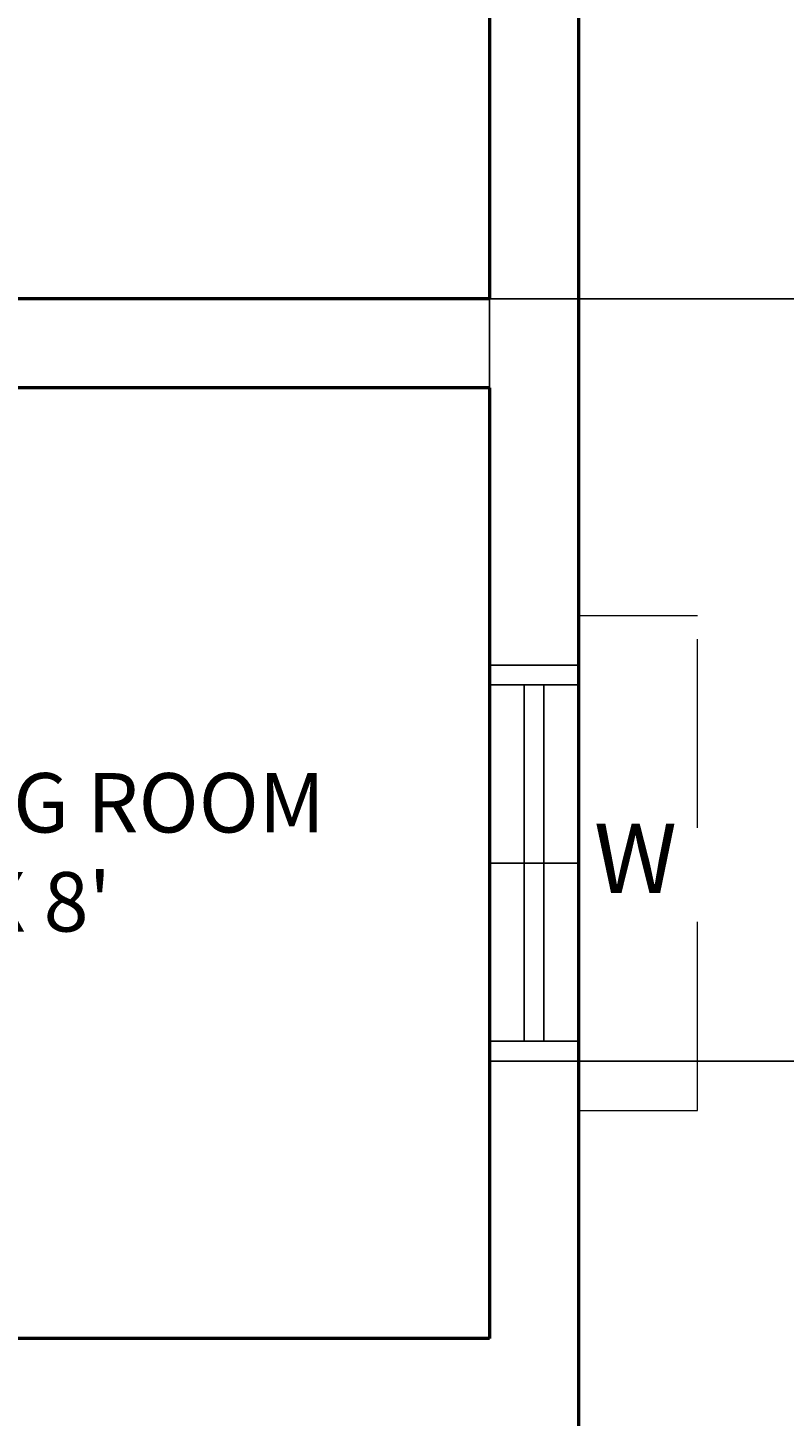
# Model space of a CAD drawing. Units: inches. Extents: x 37 to 824, y -700 to 234.
# Tile 40 of 77: x 372 to 449, y -215 to -75. Entities that reach past the tile are written whole.
import ezdxf

# ---------------------------------------------------------------- set-up
doc = ezdxf.new("R2010")
doc.units = ezdxf.units.IN
doc.header["$MEASUREMENT"] = 0
doc.linetypes.add('DASHED', pattern=[19.05, 12.7, -6.35])
for name, color, linetype, lineweight in [('A-ANNO-DIMS', 2, 'Continuous', 18), ('A-ANNO-TEXT', 7, 'Continuous', 18), ('A-AREA-IDEN', 3, 'Continuous', 18), ('A-GLAZ', 4, 'Continuous', 25), ('A-ROOF-OVHD', 1, 'DASHED', 18), ('A-WALL', 2, 'Continuous', 50)]:
    doc.layers.add(name, color=color, linetype=linetype, lineweight=lineweight)
doc.styles.get("Standard").update_dxf_attribs({"font": 'arial.ttf'})
doc.dimstyles.get("Standard").update_dxf_attribs({"dimtxt": 0.18, "dimasz": 0.18, "dimexe": 0.18, "dimexo": 0.0625, "dimgap": 0.09, "dimtad": 0, "dimtih": 1, "dimtoh": 1, "dimdec": 1, "dimzin": 0, "dimdsep": 46, "dimlunit": 4, "dimtxsty": 'Standard', "dimcen": 0.09, "dimadec": 0, "dimazin": 0, "dimtfac": 1, "dimtdec": 1, "dimtofl": 0, "dimtmove": 0, "dimatfit": 3, "dimfxl": 1, "dimtolj": 1, "dimtzin": 0, "dimarcsym": 0})

# ---------------------------------------------------------------- blocks, each defined once
blk = doc.blocks.new('WIN-900')
for p, q in [((0, 9), (0, 0)), ((2, 9), (2, 0)), ((20, 9), (20, 0)), ((38, 9), (38, 0)), ((40, 9), (40, 0)), ((38, 5.5), (2, 5.5)), ((38, 3.5), (2, 3.5))]:
    blk.add_line(p, q)
blk = doc.blocks.new('*D64')
at = {"layer": 'A-ANNO-DIMS', "color": 0, "lineweight": -2, "ltscale": 0.5, "transparency": 16777216}
for p, q in [((428.14, 191.09), (513.77, 191.09)), ((513.59, 190.91), (513.59, -87.23)), ((513.59, -365.73), (513.59, -87.59)), ((428.14, -365.91), (513.77, -365.91))]:
    blk.add_line(p, q, dxfattribs=at)
at = {"layer": 'A-ANNO-DIMS', "color": 0, "ltscale": 0.5, "transparency": 16777216}
for points in [[(513.56, 190.91), (513.62, 190.91), (513.59, 191.09)], [(513.56, -365.73), (513.62, -365.73), (513.59, -365.91)]]:
    blk.add_solid(points, dxfattribs=at)
at = {"layer": 'Defpoints', "color": 0, "ltscale": 0.5, "transparency": 16777216}
for p in [(428.08, 191.09), (428.08, -365.91), (513.59, -365.91)]:
    blk.add_point(p, dxfattribs=at)
at = {"layer": 'A-ANNO-DIMS', "color": 0, "ltscale": 0.5, "transparency": 16777216, "insert": (513.59, -87.41), "char_height": 0.18, "attachment_point": 5}
blk.add_mtext('\\A1;46\'-5"', dxfattribs=at)
blk = doc.blocks.new('*D65')
at = {"layer": 'A-ANNO-DIMS', "color": 0, "lineweight": -2, "ltscale": 0.5, "transparency": 16777216}
for p, q in [((428.14, -178.91), (513.77, -178.91)), ((513.59, -179.09), (513.59, -272.23)), ((513.59, -365.73), (513.59, -272.59)), ((428.14, -365.91), (513.77, -365.91))]:
    blk.add_line(p, q, dxfattribs=at)
at = {"layer": 'A-ANNO-DIMS', "color": 0, "ltscale": 0.5, "transparency": 16777216}
for points in [[(513.56, -179.09), (513.62, -179.09), (513.59, -178.91)], [(513.56, -365.73), (513.62, -365.73), (513.59, -365.91)]]:
    blk.add_solid(points, dxfattribs=at)
at = {"layer": 'Defpoints', "color": 0, "ltscale": 0.5, "transparency": 16777216}
for p in [(428.08, -178.91), (428.08, -365.91), (513.59, -365.91)]:
    blk.add_point(p, dxfattribs=at)
at = {"layer": 'A-ANNO-DIMS', "color": 0, "ltscale": 0.5, "transparency": 16777216, "insert": (513.59, -272.41), "char_height": 0.18, "attachment_point": 5}
blk.add_mtext('\\A1;15\'-7"', dxfattribs=at)
blk = doc.blocks.new('*D79')
at = {"layer": 'A-ANNO-DIMS', "color": 0, "lineweight": -2, "ltscale": 0.5, "transparency": 16777216}
for p, q in [((299.14, -62.02), (513.77, -62.02)), ((513.59, -62.2), (513.59, -81.78)), ((513.59, -101.73), (513.59, -82.15)), ((296.14, -101.91), (513.77, -101.91))]:
    blk.add_line(p, q, dxfattribs=at)
at = {"layer": 'A-ANNO-DIMS', "color": 0, "ltscale": 0.5, "transparency": 16777216}
for points in [[(513.56, -62.2), (513.62, -62.2), (513.59, -62.02)], [(513.56, -101.73), (513.62, -101.73), (513.59, -101.91)]]:
    blk.add_solid(points, dxfattribs=at)
at = {"layer": 'Defpoints', "color": 0, "ltscale": 0.5, "transparency": 16777216}
for p in [(299.08, -62.02), (296.08, -101.91), (513.59, -101.91)]:
    blk.add_point(p, dxfattribs=at)
at = {"layer": 'A-ANNO-DIMS', "color": 0, "ltscale": 0.5, "transparency": 16777216, "insert": (513.59, -81.97), "char_height": 0.18, "attachment_point": 5}
blk.add_mtext('\\A1;3\'-4"', dxfattribs=at)
blk = doc.blocks.new('*D83')
at = {"layer": 'A-ANNO-DIMS', "color": 0, "lineweight": -2, "ltscale": 0.5, "transparency": 16777216}
for p, q in [((358.13, -206.85), (358.13, 234.17)), ((358.31, 233.99), (388.28, 233.99)), ((418.9, 233.99), (388.93, 233.99)), ((419.08, -206.85), (419.08, 234.17))]:
    blk.add_line(p, q, dxfattribs=at)
at = {"layer": 'A-ANNO-DIMS', "color": 0, "ltscale": 0.5, "transparency": 16777216}
for points in [[(358.31, 234.02), (358.31, 233.96), (358.13, 233.99)], [(418.9, 234.02), (418.9, 233.96), (419.08, 233.99)]]:
    blk.add_solid(points, dxfattribs=at)
at = {"layer": 'Defpoints', "color": 0, "ltscale": 0.5, "transparency": 16777216}
for p in [(419.08, 233.99), (358.13, -206.91), (419.08, -206.91)]:
    blk.add_point(p, dxfattribs=at)
at = {"layer": 'A-ANNO-DIMS', "color": 0, "ltscale": 0.5, "transparency": 16777216, "insert": (388.6, 233.99), "char_height": 0.18, "attachment_point": 5}
blk.add_mtext('\\A1;5\'-1"', dxfattribs=at)

msp = doc.modelspace()

# ---------------------------------------------------------------- linework, layer by layer
at = {"layer": 'A-ROOF-OVHD', "ltscale": 1.5}
for p, q in [((428.08, -138.91), (428.08, -133.91)), ((428.08, -133.91), (440.08, -133.91)), ((440.08, -183.91), (440.08, -133.91)), ((428.08, -178.91), (428.08, -183.91)), ((428.08, -183.91), (440.08, -183.91))]:
    msp.add_line(p, q, dxfattribs=at)
at = {"layer": 'A-WALL'}
for p, q in [((419.08, 6.09), (419.08, -101.91)), ((428.08, 6.09), (428.08, -110.91)), ((419.08, -101.91), (290.08, -101.91)), ((419.08, -110.91), (290.08, -110.91)), ((419.08, -110.91), (419.08, -206.91)), ((428.08, -110.91), (428.08, -215.91)), ((419.08, -206.91), (358.13, -206.91))]:
    msp.add_line(p, q, dxfattribs=at)

# ---------------------------------------------------------------- block references
at = {"layer": 'A-GLAZ', "rotation": 270.0000000000001}
msp.add_blockref('WIN-900', (419.08, -138.91), dxfattribs=at)

# ---------------------------------------------------------------- texts
at = {"layer": 'A-ANNO-TEXT'}
msp.add_text('W', height=7, dxfattribs=at).set_placement((429.63, -161.94))
at = {"layer": 'A-AREA-IDEN', "insert": (339.67, -149.82), "char_height": 6, "attachment_point": 1}
msp.add_mtext_dynamic_manual_height_columns("DRAWING ROOM\\P        10' X 8'", width=88.3217, gutter_width=1, heights=[0], dxfattribs=at)

# ---------------------------------------------------------------- dimensions: what is measured, and where the dimension line sits
at = {"layer": 'A-ANNO-DIMS', "ltscale": 0.5}
dim = msp.add_linear_dim(base=(419.0772, 233.9904), p1=(358.1323, -206.9096), p2=(419.0772, -206.9096), dimstyle='Standard', override={"dimdec": 1, "dimlfac": 1, "dimrnd": 0, "dimzin": 1, "dimdsep": 46, "dimlunit": 4, "dimfrac": 2}, dxfattribs=at)
dim.commit()
dim.dimension.update_dxf_attribs({"geometry": '*D83', "text_midpoint": (388.6047, 233.9904)})
for base, p1, p2, picture, middle in [((513.59, -365.91), (428.08, 191.09), (428.08, -365.91), '*D64', (513.59, -87.41)), ((513.59, -101.91), (299.08, -62.02), (296.08, -101.91), '*D79', (513.59, -81.97)), ((513.59, -365.91), (428.08, -178.91), (428.08, -365.91), '*D65', (513.59, -272.41))]:
    dim = msp.add_linear_dim(base=base, p1=p1, p2=p2, angle=90, dimstyle='Standard', override={"dimdec": 1, "dimlfac": 1, "dimrnd": 0, "dimzin": 1, "dimdsep": 46, "dimlunit": 4, "dimfrac": 2}, dxfattribs=at)
    dim.commit()
    dim.dimension.update_dxf_attribs({"geometry": picture, "text_midpoint": middle})

doc.saveas('drawing.dxf')
